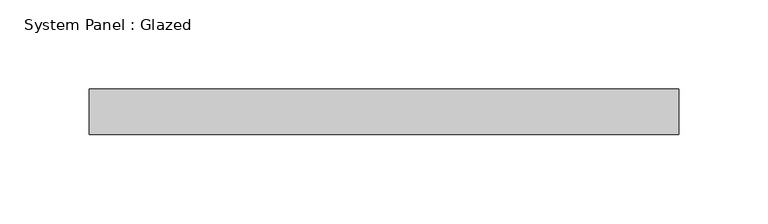
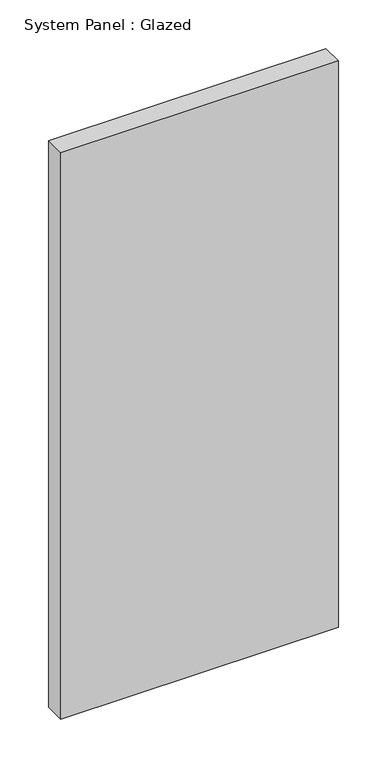
"""IFC4 building model written with IfcOpenShell, lengths in millimetres: plate geometry, System Panel : Glazed."""

from ifc_helpers import new_model, si_unit, origin, origin_with_axes, place, context, project, spatial, polyline, outline, extrude, source, transform, mapped, element, save


def system_panel_glazed_9c7248e6(model_context):
    return source(origin(), model_context, "Body", "SweptSolid", [
        extrude(outline(polyline([(165.1, 19.05), (-165.1, 19.05), (-165.1, 44.45), (165.1, 44.45), (165.1, 19.05)])), origin_with_axes(), (0.0, 0.0, 1.0), 711.7709318),
    ])


if __name__ == "__main__":
    model = new_model("IFC4")
    model_context = context("Model", 3, world=origin())
    ifc_project = project(units=[si_unit("LENGTHUNIT", "METRE", prefix="MILLI")], contexts=[model_context])
    site = spatial("IfcSite", under=ifc_project)
    building = spatial("IfcBuilding", under=site)
    placement = place(None, origin())
    system_panel_glazed_shape = system_panel_glazed_9c7248e6(model_context)
    element("IfcPlate", 1, ObjectType="System Panel : Glazed", at=placement, inside=building, context=model_context, shape_type="MappedRepresentation", body=[
        mapped(system_panel_glazed_shape, transform((0.0, 0.0, 0.0), x_axis=(1.0, 0.0, 0.0), y_axis=(0.0, 1.0, 0.0), z_axis=(0.0, 0.0, 1.0))),
    ])
    save(model, "model.ifc")

# Revit data of these elements
# Type "System Panel : Glazed"
#   Construction Type Id = "GSP4R"
#   Analytic Construction = "1/8 in Pilkington single glazing"
#   Visual Light Transmittance = 0.9
#   Solar Heat Gain Coefficient = 0.86
#   Heat Transfer Coefficient (U) = 1.18115 BTU/(h·ft²·°F)
#   Define Thermal Properties by = 1
# Element 1 (IfcPlate, "System Panel : Glazed")
#   Materials on its faces: "Glass"
# Materials
#   "Glass": class "Glass", colour RGB 0 128 192, transparency 0.75, Description = "Soda Lime Glass", Cost = 0
